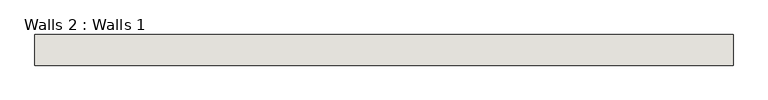
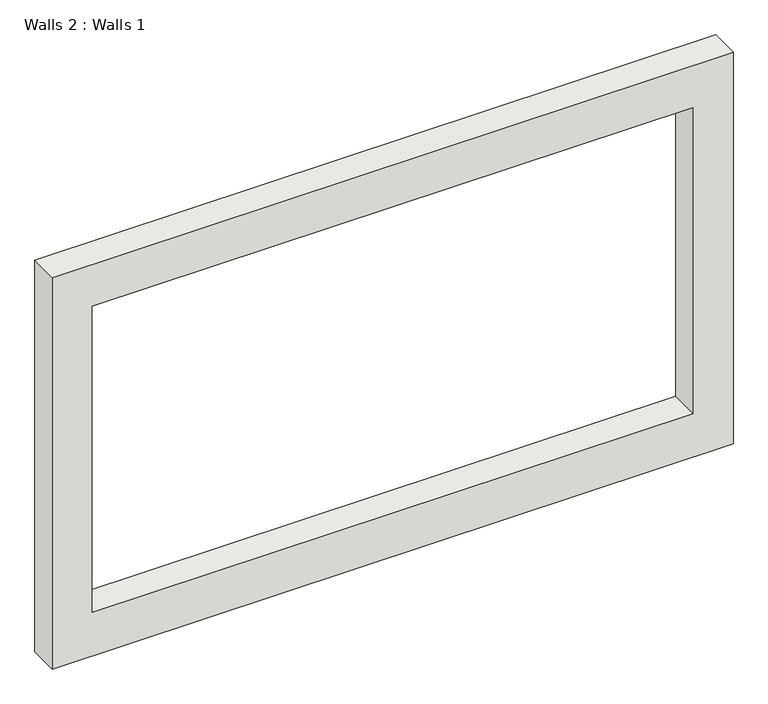
"""IFC4 building model written with IfcOpenShell, lengths in millimetres: wall geometry, Walls 2 : Walls 1."""

from ifc_helpers import new_model, si_unit, frame, origin, place, context, project, spatial, polyline, outline, extrude, source, transform, mapped, element, save


def walls_2_walls_1_3aef9765(model_context):
    return source(origin(), model_context, "Body", "SweptSolid", [
        extrude(outline(polyline([(13976.9693979, 1712.6958607), (13976.9693979, -878.1041393), (12402.1693979, -878.1041393), (12402.1693979, 1712.6958607), (13976.9693979, 1712.6958607)]), holes=[polyline([(13807.224337, 1560.0533085), (12576.3422066, 1560.0533085), (12576.3422066, -725.9466915), (13807.224337, -725.9466915), (13807.224337, 1560.0533085)])]), frame((0.0, -4102.7951319, 0.0), z_axis=(0.0, 1.0, 0.0), x_axis=(0.0, 0.0, 1.0)), (0.0, 0.0, 1.0), 113.5625565),
    ])


if __name__ == "__main__":
    model = new_model("IFC4")
    model_context = context("Model", 3, world=origin())
    ifc_project = project(units=[si_unit("LENGTHUNIT", "METRE", prefix="MILLI")], contexts=[model_context])
    site = spatial("IfcSite", under=ifc_project)
    building = spatial("IfcBuilding", under=site)
    placement = place(None, origin())
    walls_2_walls_1_shape = walls_2_walls_1_3aef9765(model_context)
    element("IfcWall", 1, ObjectType="Walls 2 : Walls 1", at=placement, inside=building, context=model_context, shape_type="MappedRepresentation", body=[
        mapped(walls_2_walls_1_shape, transform((0.0, 0.0, 0.0), x_axis=(1.0, 0.0, 0.0), y_axis=(0.0, 1.0, 0.0), z_axis=(0.0, 0.0, 1.0))),
    ])
    save(model, "model.ifc")

# Revit data of these elements
# Element 1 (IfcWall, "Walls 2 : Walls 1")
#   Materials on its faces: "Default Wall"
# Materials
#   "Default Wall": colour RGB 128 128 128, transparency 0
